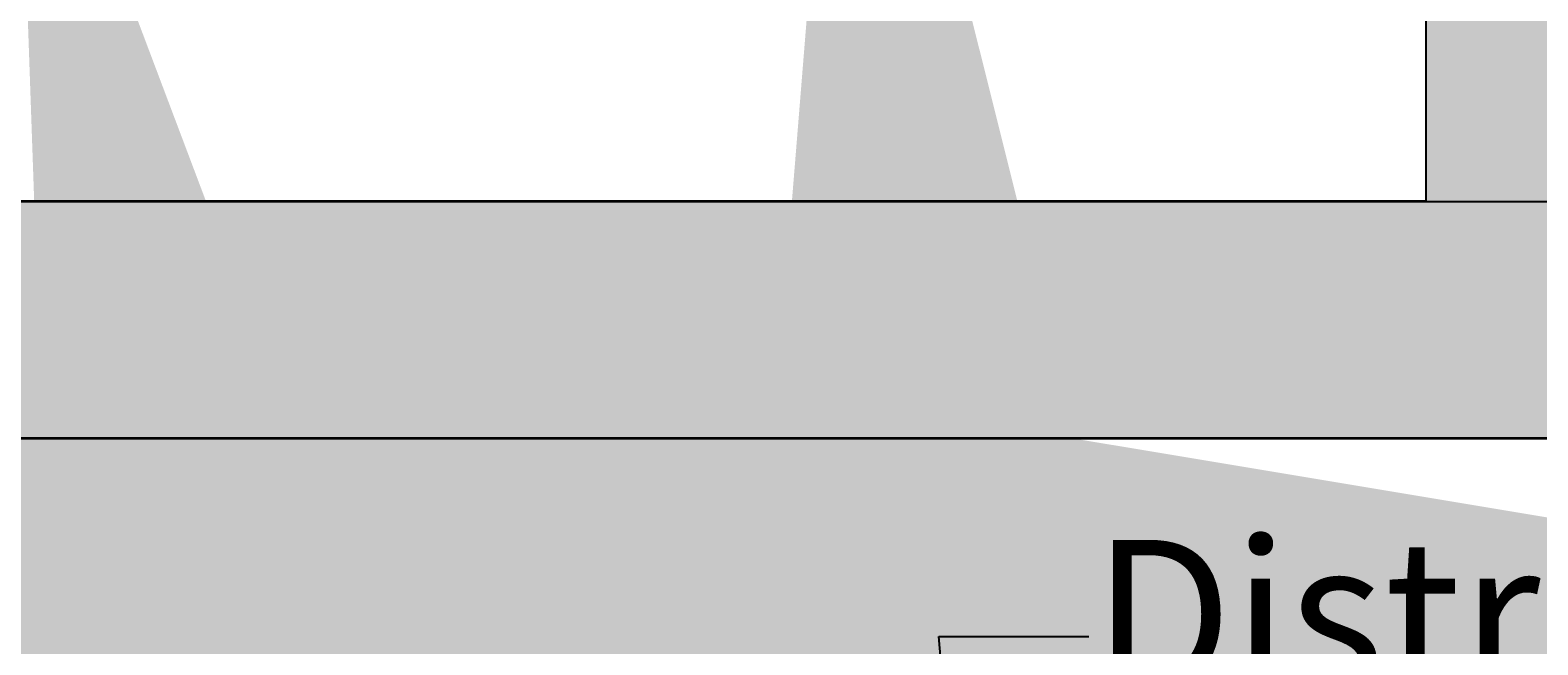
# Model space of a CAD drawing. Units: millimetres. Extents: x -22994 to 29398, y -19990 to 20176.
# Tile 13 of 135: x 58 to 99, y 5 to 21. Entities that reach past the tile are written whole.
import ezdxf
from ezdxf import colors
from ezdxf.entities.mleader import LeaderData, LeaderLine
from ezdxf.math import Vec2, Vec3

# ---------------------------------------------------------------- set-up
doc = ezdxf.new("R2010")
doc.units = ezdxf.units.MM
doc.header["$MEASUREMENT"] = 0
for name, color, linetype, lineweight in [('M-ANNO-TEXT', 7, 'Continuous', 25), ('M-DIMS', 2, 'Continuous', 18), ('M-EQPM', 7, 'Continuous', 25), ('M-EQPM-PATT', 7, 'Continuous', 18), ('S-FNDN', 7, 'Continuous', 35)]:
    doc.layers.add(name, color=color, linetype=linetype, lineweight=lineweight)
doc.styles.get("Standard").update_dxf_attribs({"font": 'arial.ttf'})
doc.dimstyles.get("Standard").update_dxf_attribs({"dimtxt": 0.18, "dimasz": 10000, "dimexe": 0.18, "dimexo": 0.0625, "dimgap": 0.09, "dimtad": 0, "dimtih": 1, "dimtoh": 1, "dimdec": 0, "dimzin": 0, "dimdsep": 46, "dimtxsty": 'Standard', "dimcen": 0.09, "dimadec": 0, "dimazin": 0, "dimtfac": 1, "dimtdec": 0, "dimtofl": 0, "dimtmove": 0, "dimatfit": 3, "dimfxl": 1, "dimtolj": 1, "dimtzin": 0, "dimlwd": 30, "dimarcsym": 0})

# ---------------------------------------------------------------- blocks, each defined once
blk = doc.blocks.new('*D2')
at = {"layer": 'Defpoints', "color": 0, "transparency": 16777216}
for p in [(6.677, 10.271), (290.852, 10.271), (290.852, -5.079)]:
    blk.add_point(p, dxfattribs=at)
at = {"layer": 'M-DIMS', "color": 0, "lineweight": -2, "transparency": 16777216}
for p, q in [((6.677, 10.209), (6.677, -5.259)), ((290.852, 10.209), (290.852, -5.259))]:
    blk.add_line(p, q, dxfattribs=at)
at = {"layer": 'M-DIMS', "color": 0, "lineweight": 30, "transparency": 16777216}
for p, q in [((-9993.323, -5.079), (-19993.323, -5.079)), ((10290.852, -5.079), (20290.852, -5.079))]:
    blk.add_line(p, q, dxfattribs=at)
at = {"layer": 'M-DIMS', "color": 0, "transparency": 16777216}
for points in [[(-9993.323, 1661.588), (-9993.323, -1671.745), (6.677, -5.079)], [(10290.852, 1661.588), (10290.852, -1671.745), (290.852, -5.079)]]:
    blk.add_solid(points, dxfattribs=at)
at = {"layer": 'M-DIMS', "color": 0, "transparency": 16777216, "insert": (148.765, -5.079), "char_height": 0.18, "attachment_point": 5}
blk.add_mtext('\\A1;284.2', dxfattribs=at)
blk = doc.blocks.new('*D3')
at = {"layer": 'Defpoints', "color": 0, "transparency": 16777216}
for p in [(110.265, 204.165), (110.265, 176.366), (95.833, 127.967)]:
    blk.add_point(p, dxfattribs=at)
at = {"layer": 'M-DIMS', "color": 0, "lineweight": 30, "transparency": 16777216}
for p, q in [((-9904.167, 204.165), (-19904.167, 204.165)), ((10110.265, 204.165), (20110.265, 204.165))]:
    blk.add_line(p, q, dxfattribs=at)
at = {"layer": 'M-DIMS', "color": 0, "lineweight": -2, "transparency": 16777216}
for p, q in [((95.833, 128.03), (95.833, 204.345)), ((110.265, 176.429), (110.265, 204.345))]:
    blk.add_line(p, q, dxfattribs=at)
at = {"layer": 'M-DIMS', "color": 0, "transparency": 16777216}
for points in [[(-9904.167, 1870.832), (-9904.167, -1462.501), (95.833, 204.165)], [(10110.265, 1870.832), (10110.265, -1462.501), (110.265, 204.165)]]:
    blk.add_solid(points, dxfattribs=at)
at = {"layer": 'M-DIMS', "color": 0, "transparency": 16777216, "insert": (103.049, 204.165), "char_height": 0.18, "attachment_point": 5}
blk.add_mtext('\\A1;14.432', dxfattribs=at)
blk = doc.blocks.new('*D4')
at = {"layer": 'Defpoints', "color": 0, "transparency": 16777216}
for p in [(116.265, 204.165), (110.265, 176.366), (116.265, 176.366)]:
    blk.add_point(p, dxfattribs=at)
at = {"layer": 'M-DIMS', "color": 0, "lineweight": 30, "transparency": 16777216}
for p, q in [((-9889.735, 204.165), (-19889.735, 204.165)), ((10116.265, 204.165), (20116.265, 204.165))]:
    blk.add_line(p, q, dxfattribs=at)
at = {"layer": 'M-DIMS', "color": 0, "lineweight": -2, "transparency": 16777216}
for p, q in [((110.265, 176.429), (110.265, 204.345)), ((116.265, 176.429), (116.265, 204.345))]:
    blk.add_line(p, q, dxfattribs=at)
at = {"layer": 'M-DIMS', "color": 0, "transparency": 16777216}
for points in [[(-9889.735, 1870.832), (-9889.735, -1462.501), (110.265, 204.165)], [(10116.265, 1870.832), (10116.265, -1462.501), (116.265, 204.165)]]:
    blk.add_solid(points, dxfattribs=at)
at = {"layer": 'M-DIMS', "color": 0, "transparency": 16777216, "insert": (113.265, 204.165), "char_height": 0.18, "attachment_point": 5}
blk.add_mtext('\\A1;6', dxfattribs=at)
blk = doc.blocks.new('*D5')
at = {"layer": 'Defpoints', "color": 0, "transparency": 16777216}
for p in [(181.265, 204.165), (116.265, 176.366), (181.265, 176.366)]:
    blk.add_point(p, dxfattribs=at)
at = {"layer": 'M-DIMS', "color": 0, "lineweight": 30, "transparency": 16777216}
for p, q in [((-9883.735, 204.165), (-19883.735, 204.165)), ((10181.265, 204.165), (20181.265, 204.165))]:
    blk.add_line(p, q, dxfattribs=at)
at = {"layer": 'M-DIMS', "color": 0, "lineweight": -2, "transparency": 16777216}
for p, q in [((116.265, 176.429), (116.265, 204.345)), ((181.265, 176.429), (181.265, 204.345))]:
    blk.add_line(p, q, dxfattribs=at)
at = {"layer": 'M-DIMS', "color": 0, "transparency": 16777216}
for points in [[(-9883.735, 1870.832), (-9883.735, -1462.501), (116.265, 204.165)], [(10181.265, 1870.832), (10181.265, -1462.501), (181.265, 204.165)]]:
    blk.add_solid(points, dxfattribs=at)
at = {"layer": 'M-DIMS', "color": 0, "transparency": 16777216, "insert": (148.765, 204.165), "char_height": 0.18, "attachment_point": 5}
blk.add_mtext('\\A1;65', dxfattribs=at)
blk = doc.blocks.new('*D6')
at = {"layer": 'Defpoints', "color": 0, "transparency": 16777216}
for p in [(187.265, 204.165), (181.265, 176.366), (187.265, 176.366)]:
    blk.add_point(p, dxfattribs=at)
at = {"layer": 'M-DIMS', "color": 0, "lineweight": 30, "transparency": 16777216}
for p, q in [((-9818.735, 204.165), (-19818.735, 204.165)), ((10187.265, 204.165), (20187.265, 204.165))]:
    blk.add_line(p, q, dxfattribs=at)
at = {"layer": 'M-DIMS', "color": 0, "lineweight": -2, "transparency": 16777216}
for p, q in [((181.265, 176.429), (181.265, 204.345)), ((187.265, 176.429), (187.265, 204.345))]:
    blk.add_line(p, q, dxfattribs=at)
at = {"layer": 'M-DIMS', "color": 0, "transparency": 16777216}
for points in [[(-9818.735, 1870.832), (-9818.735, -1462.501), (181.265, 204.165)], [(10187.265, 1870.832), (10187.265, -1462.501), (187.265, 204.165)]]:
    blk.add_solid(points, dxfattribs=at)
at = {"layer": 'M-DIMS', "color": 0, "transparency": 16777216, "insert": (184.265, 204.165), "char_height": 0.18, "attachment_point": 5}
blk.add_mtext('\\A1;6', dxfattribs=at)
blk = doc.blocks.new('*D7')
at = {"layer": 'Defpoints', "color": 0, "transparency": 16777216}
for p in [(201.697, 204.165), (187.265, 176.366), (201.697, 127.967)]:
    blk.add_point(p, dxfattribs=at)
at = {"layer": 'M-DIMS', "color": 0, "lineweight": 30, "transparency": 16777216}
for p, q in [((-9812.735, 204.165), (-19812.735, 204.165)), ((10201.697, 204.165), (20201.697, 204.165))]:
    blk.add_line(p, q, dxfattribs=at)
at = {"layer": 'M-DIMS', "color": 0, "lineweight": -2, "transparency": 16777216}
for p, q in [((187.265, 176.429), (187.265, 204.345)), ((201.697, 128.03), (201.697, 204.345))]:
    blk.add_line(p, q, dxfattribs=at)
at = {"layer": 'M-DIMS', "color": 0, "transparency": 16777216}
for points in [[(-9812.735, 1870.832), (-9812.735, -1462.501), (187.265, 204.165)], [(10201.697, 1870.832), (10201.697, -1462.501), (201.697, 204.165)]]:
    blk.add_solid(points, dxfattribs=at)
at = {"layer": 'M-DIMS', "color": 0, "transparency": 16777216, "insert": (194.481, 204.165), "char_height": 0.18, "attachment_point": 5}
blk.add_mtext('\\A1;14.432', dxfattribs=at)
blk = doc.blocks.new('*D8')
at = {"layer": 'Defpoints', "color": 0, "transparency": 16777216}
for p in [(227.648, 204.165), (227.648, 146.73), (201.697, 127.967)]:
    blk.add_point(p, dxfattribs=at)
at = {"layer": 'M-DIMS', "color": 0, "lineweight": 30, "transparency": 16777216}
for p, q in [((-9798.303, 204.165), (-19798.303, 204.165)), ((10227.648, 204.165), (20227.648, 204.165))]:
    blk.add_line(p, q, dxfattribs=at)
at = {"layer": 'M-DIMS', "color": 0, "lineweight": -2, "transparency": 16777216}
for p, q in [((201.697, 128.03), (201.697, 204.345)), ((227.648, 146.792), (227.648, 204.345))]:
    blk.add_line(p, q, dxfattribs=at)
at = {"layer": 'M-DIMS', "color": 0, "transparency": 16777216}
for points in [[(-9798.303, 1870.832), (-9798.303, -1462.501), (201.697, 204.165)], [(10227.648, 1870.832), (10227.648, -1462.501), (227.648, 204.165)]]:
    blk.add_solid(points, dxfattribs=at)
at = {"layer": 'M-DIMS', "color": 0, "transparency": 16777216, "insert": (214.673, 204.165), "char_height": 0.18, "attachment_point": 5}
blk.add_mtext('\\A1;25.95', dxfattribs=at)
blk = doc.blocks.new('*D9')
at = {"layer": 'Defpoints', "color": 0, "transparency": 16777216}
for p in [(187.265, 176.366), (306.202, 176.366), (290.852, 10.271)]:
    blk.add_point(p, dxfattribs=at)
at = {"layer": 'M-DIMS', "color": 0, "lineweight": 30, "transparency": 16777216}
for p, q in [((306.202, 10176.366), (306.202, 20176.366)), ((306.202, -9989.729), (306.202, -19989.729))]:
    blk.add_line(p, q, dxfattribs=at)
at = {"layer": 'M-DIMS', "color": 0, "lineweight": -2, "transparency": 16777216}
for p, q in [((187.327, 176.366), (306.382, 176.366)), ((290.915, 10.271), (306.382, 10.271))]:
    blk.add_line(p, q, dxfattribs=at)
at = {"layer": 'M-DIMS', "color": 0, "transparency": 16777216}
for points in [[(-1360.465, 10176.366), (1972.869, 10176.366), (306.202, 176.366)], [(-1360.465, -9989.729), (1972.869, -9989.729), (306.202, 10.271)]]:
    blk.add_solid(points, dxfattribs=at)
at = {"layer": 'M-DIMS', "color": 0, "transparency": 16777216, "insert": (306.202, 93.319), "char_height": 0.18, "attachment_point": 5}
blk.add_mtext('\\A1;166.1', dxfattribs=at)
blk = doc.blocks.new('*D10')
at = {"layer": 'Defpoints', "color": 0, "transparency": 16777216}
for p in [(125.65, 136.071), (133.346, 136.071), (133.346, -5.079)]:
    blk.add_point(p, dxfattribs=at)
at = {"layer": 'M-DIMS', "color": 0, "lineweight": -2, "transparency": 16777216}
for p, q in [((125.65, 136.009), (125.65, -5.259)), ((133.346, 136.009), (133.346, -5.259))]:
    blk.add_line(p, q, dxfattribs=at)
at = {"layer": 'M-DIMS', "color": 0, "lineweight": 30, "transparency": 16777216}
for p, q in [((-9874.35, -5.079), (-19874.35, -5.079)), ((10133.346, -5.079), (20133.346, -5.079))]:
    blk.add_line(p, q, dxfattribs=at)
at = {"layer": 'M-DIMS', "color": 0, "transparency": 16777216}
for points in [[(-9874.35, 1661.588), (-9874.35, -1671.745), (125.65, -5.079)], [(10133.346, 1661.588), (10133.346, -1671.745), (133.346, -5.079)]]:
    blk.add_solid(points, dxfattribs=at)
at = {"layer": 'M-DIMS', "color": 0, "transparency": 16777216, "insert": (129.498, -5.079), "char_height": 0.18, "attachment_point": 5}
blk.add_mtext('\\A1;7.696', dxfattribs=at)
blk = doc.blocks.new('*D11')
at = {"layer": 'Defpoints', "color": 0, "transparency": 16777216}
for p in [(133.346, 136.071), (135.65, 136.071), (135.65, -5.079)]:
    blk.add_point(p, dxfattribs=at)
at = {"layer": 'M-DIMS', "color": 0, "lineweight": -2, "transparency": 16777216}
for p, q in [((133.346, 136.009), (133.346, -5.259)), ((135.65, 136.009), (135.65, -5.259))]:
    blk.add_line(p, q, dxfattribs=at)
at = {"layer": 'M-DIMS', "color": 0, "lineweight": 30, "transparency": 16777216}
for p, q in [((-9866.654, -5.079), (-19866.654, -5.079)), ((10135.65, -5.079), (20135.65, -5.079))]:
    blk.add_line(p, q, dxfattribs=at)
at = {"layer": 'M-DIMS', "color": 0, "transparency": 16777216}
for points in [[(-9866.654, 1661.588), (-9866.654, -1671.745), (133.346, -5.079)], [(10135.65, 1661.588), (10135.65, -1671.745), (135.65, -5.079)]]:
    blk.add_solid(points, dxfattribs=at)
at = {"layer": 'M-DIMS', "color": 0, "transparency": 16777216, "insert": (134.498, -5.079), "char_height": 0.18, "attachment_point": 5}
blk.add_mtext('\\A1;2.304', dxfattribs=at)
blk = doc.blocks.new('*D12')
at = {"layer": 'Defpoints', "color": 0, "transparency": 16777216}
for p in [(135.65, 136.071), (145.65, 136.071), (145.65, -5.079)]:
    blk.add_point(p, dxfattribs=at)
at = {"layer": 'M-DIMS', "color": 0, "lineweight": -2, "transparency": 16777216}
for p, q in [((135.65, 136.009), (135.65, -5.259)), ((145.65, 136.009), (145.65, -5.259))]:
    blk.add_line(p, q, dxfattribs=at)
at = {"layer": 'M-DIMS', "color": 0, "lineweight": 30, "transparency": 16777216}
for p, q in [((-9864.35, -5.079), (-19864.35, -5.079)), ((10145.65, -5.079), (20145.65, -5.079))]:
    blk.add_line(p, q, dxfattribs=at)
at = {"layer": 'M-DIMS', "color": 0, "transparency": 16777216}
for points in [[(-9864.35, 1661.588), (-9864.35, -1671.745), (135.65, -5.079)], [(10145.65, 1661.588), (10145.65, -1671.745), (145.65, -5.079)]]:
    blk.add_solid(points, dxfattribs=at)
at = {"layer": 'M-DIMS', "color": 0, "transparency": 16777216, "insert": (140.65, -5.079), "char_height": 0.18, "attachment_point": 5}
blk.add_mtext('\\A1;10', dxfattribs=at)
blk = doc.blocks.new('*D13')
at = {"layer": 'Defpoints', "color": 0, "transparency": 16777216}
for p in [(145.65, 136.071), (155.65, 136.071), (155.65, -5.079)]:
    blk.add_point(p, dxfattribs=at)
at = {"layer": 'M-DIMS', "color": 0, "lineweight": -2, "transparency": 16777216}
for p, q in [((145.65, 136.009), (145.65, -5.259)), ((155.65, 136.009), (155.65, -5.259))]:
    blk.add_line(p, q, dxfattribs=at)
at = {"layer": 'M-DIMS', "color": 0, "lineweight": 30, "transparency": 16777216}
for p, q in [((-9854.35, -5.079), (-19854.35, -5.079)), ((10155.65, -5.079), (20155.65, -5.079))]:
    blk.add_line(p, q, dxfattribs=at)
at = {"layer": 'M-DIMS', "color": 0, "transparency": 16777216}
for points in [[(-9854.35, 1661.588), (-9854.35, -1671.745), (145.65, -5.079)], [(10155.65, 1661.588), (10155.65, -1671.745), (155.65, -5.079)]]:
    blk.add_solid(points, dxfattribs=at)
at = {"layer": 'M-DIMS', "color": 0, "transparency": 16777216, "insert": (150.65, -5.079), "char_height": 0.18, "attachment_point": 5}
blk.add_mtext('\\A1;10', dxfattribs=at)
blk = doc.blocks.new('*D14')
at = {"layer": 'Defpoints', "color": 0, "transparency": 16777216}
for p in [(155.65, 136.071), (165.65, 136.071), (165.65, -5.079)]:
    blk.add_point(p, dxfattribs=at)
at = {"layer": 'M-DIMS', "color": 0, "lineweight": -2, "transparency": 16777216}
for p, q in [((155.65, 136.009), (155.65, -5.259)), ((165.65, 136.009), (165.65, -5.259))]:
    blk.add_line(p, q, dxfattribs=at)
at = {"layer": 'M-DIMS', "color": 0, "lineweight": 30, "transparency": 16777216}
for p, q in [((-9844.35, -5.079), (-19844.35, -5.079)), ((10165.65, -5.079), (20165.65, -5.079))]:
    blk.add_line(p, q, dxfattribs=at)
at = {"layer": 'M-DIMS', "color": 0, "transparency": 16777216}
for points in [[(-9844.35, 1661.588), (-9844.35, -1671.745), (155.65, -5.079)], [(10165.65, 1661.588), (10165.65, -1671.745), (165.65, -5.079)]]:
    blk.add_solid(points, dxfattribs=at)
at = {"layer": 'M-DIMS', "color": 0, "transparency": 16777216, "insert": (160.65, -5.079), "char_height": 0.18, "attachment_point": 5}
blk.add_mtext('\\A1;10', dxfattribs=at)
blk = doc.blocks.new('*D15')
at = {"layer": 'Defpoints', "color": 0, "transparency": 16777216}
for p in [(173.346, 154.788), (173.346, 136.071), (306.202, 136.071)]:
    blk.add_point(p, dxfattribs=at)
at = {"layer": 'M-DIMS', "color": 0, "lineweight": 30, "transparency": 16777216}
for p, q in [((306.202, 10154.788), (306.202, 20154.788)), ((306.202, -9863.929), (306.202, -19863.929))]:
    blk.add_line(p, q, dxfattribs=at)
at = {"layer": 'M-DIMS', "color": 0, "lineweight": -2, "transparency": 16777216}
for p, q in [((173.408, 154.788), (306.382, 154.788)), ((173.408, 136.071), (306.382, 136.071))]:
    blk.add_line(p, q, dxfattribs=at)
at = {"layer": 'M-DIMS', "color": 0, "transparency": 16777216}
for points in [[(-1360.465, 10154.788), (1972.869, 10154.788), (306.202, 154.788)], [(-1360.465, -9863.929), (1972.869, -9863.929), (306.202, 136.071)]]:
    blk.add_solid(points, dxfattribs=at)
at = {"layer": 'M-DIMS', "color": 0, "transparency": 16777216, "insert": (306.202, 145.43), "char_height": 0.18, "attachment_point": 5}
blk.add_mtext('\\A1;18.717', dxfattribs=at)
blk = doc.blocks.new('*D16')
at = {"layer": 'Defpoints', "color": 0, "transparency": 16777216}
for p in [(120.17, 204.165), (110.466, 48.035), (120.17, 48.035)]:
    blk.add_point(p, dxfattribs=at)
at = {"layer": 'M-DIMS', "color": 0, "lineweight": 30, "transparency": 16777216}
for p, q in [((-9889.534, 204.165), (-19889.534, 204.165)), ((10120.17, 204.165), (20120.17, 204.165))]:
    blk.add_line(p, q, dxfattribs=at)
at = {"layer": 'M-DIMS', "color": 0, "lineweight": -2, "transparency": 16777216}
for p, q in [((110.466, 48.097), (110.466, 204.345)), ((120.17, 48.097), (120.17, 204.345))]:
    blk.add_line(p, q, dxfattribs=at)
at = {"layer": 'M-DIMS', "color": 0, "transparency": 16777216}
for points in [[(-9889.534, 1870.832), (-9889.534, -1462.501), (110.466, 204.165)], [(10120.17, 1870.832), (10120.17, -1462.501), (120.17, 204.165)]]:
    blk.add_solid(points, dxfattribs=at)
at = {"layer": 'M-DIMS', "color": 0, "transparency": 16777216, "insert": (115.318, 204.165), "char_height": 0.18, "attachment_point": 5}
blk.add_mtext('\\A1;9.704', dxfattribs=at)
blk = doc.blocks.new('*D17')
at = {"layer": 'Defpoints', "color": 0, "transparency": 16777216}
for p in [(126.17, 204.165), (120.17, 48.035), (126.17, 48.035)]:
    blk.add_point(p, dxfattribs=at)
at = {"layer": 'M-DIMS', "color": 0, "lineweight": 30, "transparency": 16777216}
for p, q in [((-9879.83, 204.165), (-19879.83, 204.165)), ((10126.17, 204.165), (20126.17, 204.165))]:
    blk.add_line(p, q, dxfattribs=at)
at = {"layer": 'M-DIMS', "color": 0, "lineweight": -2, "transparency": 16777216}
for p, q in [((120.17, 48.097), (120.17, 204.345)), ((126.17, 48.097), (126.17, 204.345))]:
    blk.add_line(p, q, dxfattribs=at)
at = {"layer": 'M-DIMS', "color": 0, "transparency": 16777216}
for points in [[(-9879.83, 1870.832), (-9879.83, -1462.501), (120.17, 204.165)], [(10126.17, 1870.832), (10126.17, -1462.501), (126.17, 204.165)]]:
    blk.add_solid(points, dxfattribs=at)
at = {"layer": 'M-DIMS', "color": 0, "transparency": 16777216, "insert": (123.17, 204.165), "char_height": 0.18, "attachment_point": 5}
blk.add_mtext('\\A1;6', dxfattribs=at)
blk = doc.blocks.new('*D18')
at = {"layer": 'Defpoints', "color": 0, "transparency": 16777216}
for p in [(132.17, 204.165), (126.17, 48.035), (132.17, 48.035)]:
    blk.add_point(p, dxfattribs=at)
at = {"layer": 'M-DIMS', "color": 0, "lineweight": 30, "transparency": 16777216}
for p, q in [((-9873.83, 204.165), (-19873.83, 204.165)), ((10132.17, 204.165), (20132.17, 204.165))]:
    blk.add_line(p, q, dxfattribs=at)
at = {"layer": 'M-DIMS', "color": 0, "lineweight": -2, "transparency": 16777216}
for p, q in [((126.17, 48.097), (126.17, 204.345)), ((132.17, 48.097), (132.17, 204.345))]:
    blk.add_line(p, q, dxfattribs=at)
at = {"layer": 'M-DIMS', "color": 0, "transparency": 16777216}
for points in [[(-9873.83, 1870.832), (-9873.83, -1462.501), (126.17, 204.165)], [(10132.17, 1870.832), (10132.17, -1462.501), (132.17, 204.165)]]:
    blk.add_solid(points, dxfattribs=at)
at = {"layer": 'M-DIMS', "color": 0, "transparency": 16777216, "insert": (129.17, 204.165), "char_height": 0.18, "attachment_point": 5}
blk.add_mtext('\\A1;6', dxfattribs=at)
blk = doc.blocks.new('*D19')
at = {"layer": 'Defpoints', "color": 0, "transparency": 16777216}
for p in [(138.17, 204.165), (132.17, 48.035), (138.17, 48.035)]:
    blk.add_point(p, dxfattribs=at)
at = {"layer": 'M-DIMS', "color": 0, "lineweight": 30, "transparency": 16777216}
for p, q in [((-9867.83, 204.165), (-19867.83, 204.165)), ((10138.17, 204.165), (20138.17, 204.165))]:
    blk.add_line(p, q, dxfattribs=at)
at = {"layer": 'M-DIMS', "color": 0, "lineweight": -2, "transparency": 16777216}
for p, q in [((132.17, 48.097), (132.17, 204.345)), ((138.17, 48.097), (138.17, 204.345))]:
    blk.add_line(p, q, dxfattribs=at)
at = {"layer": 'M-DIMS', "color": 0, "transparency": 16777216}
for points in [[(-9867.83, 1870.832), (-9867.83, -1462.501), (132.17, 204.165)], [(10138.17, 1870.832), (10138.17, -1462.501), (138.17, 204.165)]]:
    blk.add_solid(points, dxfattribs=at)
at = {"layer": 'M-DIMS', "color": 0, "transparency": 16777216, "insert": (135.17, 204.165), "char_height": 0.18, "attachment_point": 5}
blk.add_mtext('\\A1;6', dxfattribs=at)
blk = doc.blocks.new('*D20')
at = {"layer": 'Defpoints', "color": 0, "transparency": 16777216}
for p in [(144.17, 204.165), (138.17, 48.035), (144.17, 48.035)]:
    blk.add_point(p, dxfattribs=at)
at = {"layer": 'M-DIMS', "color": 0, "lineweight": 30, "transparency": 16777216}
for p, q in [((-9861.83, 204.165), (-19861.83, 204.165)), ((10144.17, 204.165), (20144.17, 204.165))]:
    blk.add_line(p, q, dxfattribs=at)
at = {"layer": 'M-DIMS', "color": 0, "lineweight": -2, "transparency": 16777216}
for p, q in [((138.17, 48.097), (138.17, 204.345)), ((144.17, 48.097), (144.17, 204.345))]:
    blk.add_line(p, q, dxfattribs=at)
at = {"layer": 'M-DIMS', "color": 0, "transparency": 16777216}
for points in [[(-9861.83, 1870.832), (-9861.83, -1462.501), (138.17, 204.165)], [(10144.17, 1870.832), (10144.17, -1462.501), (144.17, 204.165)]]:
    blk.add_solid(points, dxfattribs=at)
at = {"layer": 'M-DIMS', "color": 0, "transparency": 16777216, "insert": (141.17, 204.165), "char_height": 0.18, "attachment_point": 5}
blk.add_mtext('\\A1;6', dxfattribs=at)
blk = doc.blocks.new('*D21')
at = {"layer": 'Defpoints', "color": 0, "transparency": 16777216}
for p in [(149.116, 204.165), (144.17, 48.035), (149.116, 48.035)]:
    blk.add_point(p, dxfattribs=at)
at = {"layer": 'M-DIMS', "color": 0, "lineweight": 30, "transparency": 16777216}
for p, q in [((-9855.83, 204.165), (-19855.83, 204.165)), ((10149.116, 204.165), (20149.116, 204.165))]:
    blk.add_line(p, q, dxfattribs=at)
at = {"layer": 'M-DIMS', "color": 0, "lineweight": -2, "transparency": 16777216}
for p, q in [((144.17, 48.097), (144.17, 204.345)), ((149.116, 48.097), (149.116, 204.345))]:
    blk.add_line(p, q, dxfattribs=at)
at = {"layer": 'M-DIMS', "color": 0, "transparency": 16777216}
for points in [[(-9855.83, 1870.832), (-9855.83, -1462.501), (144.17, 204.165)], [(10149.116, 1870.832), (10149.116, -1462.501), (149.116, 204.165)]]:
    blk.add_solid(points, dxfattribs=at)
at = {"layer": 'M-DIMS', "color": 0, "transparency": 16777216, "insert": (146.643, 204.165), "char_height": 0.18, "attachment_point": 5}
blk.add_mtext('\\A1;4.945', dxfattribs=at)
blk = doc.blocks.new('*D22')
at = {"layer": 'Defpoints', "color": 0, "transparency": 16777216}
for p in [(149.116, 30.99), (155.116, 30.99), (155.116, -5.079)]:
    blk.add_point(p, dxfattribs=at)
at = {"layer": 'M-DIMS', "color": 0, "lineweight": -2, "transparency": 16777216}
for p, q in [((149.116, 30.927), (149.116, -5.259)), ((155.116, 30.927), (155.116, -5.259))]:
    blk.add_line(p, q, dxfattribs=at)
at = {"layer": 'M-DIMS', "color": 0, "lineweight": 30, "transparency": 16777216}
for p, q in [((-9850.884, -5.079), (-19850.884, -5.079)), ((10155.116, -5.079), (20155.116, -5.079))]:
    blk.add_line(p, q, dxfattribs=at)
at = {"layer": 'M-DIMS', "color": 0, "transparency": 16777216}
for points in [[(-9850.884, 1661.588), (-9850.884, -1671.745), (149.116, -5.079)], [(10155.116, 1661.588), (10155.116, -1671.745), (155.116, -5.079)]]:
    blk.add_solid(points, dxfattribs=at)
at = {"layer": 'M-DIMS', "color": 0, "transparency": 16777216, "insert": (152.116, -5.079), "char_height": 0.18, "attachment_point": 5}
blk.add_mtext('\\A1;6', dxfattribs=at)
blk = doc.blocks.new('*D23')
at = {"layer": 'Defpoints', "color": 0, "transparency": 16777216}
for p in [(155.116, 30.99), (161.116, 30.99), (161.116, -5.079)]:
    blk.add_point(p, dxfattribs=at)
at = {"layer": 'M-DIMS', "color": 0, "lineweight": -2, "transparency": 16777216}
for p, q in [((155.116, 30.927), (155.116, -5.259)), ((161.116, 30.927), (161.116, -5.259))]:
    blk.add_line(p, q, dxfattribs=at)
at = {"layer": 'M-DIMS', "color": 0, "lineweight": 30, "transparency": 16777216}
for p, q in [((-9844.884, -5.079), (-19844.884, -5.079)), ((10161.116, -5.079), (20161.116, -5.079))]:
    blk.add_line(p, q, dxfattribs=at)
at = {"layer": 'M-DIMS', "color": 0, "transparency": 16777216}
for points in [[(-9844.884, 1661.588), (-9844.884, -1671.745), (155.116, -5.079)], [(10161.116, 1661.588), (10161.116, -1671.745), (161.116, -5.079)]]:
    blk.add_solid(points, dxfattribs=at)
at = {"layer": 'M-DIMS', "color": 0, "transparency": 16777216, "insert": (158.116, -5.079), "char_height": 0.18, "attachment_point": 5}
blk.add_mtext('\\A1;6', dxfattribs=at)
blk = doc.blocks.new('*D24')
at = {"layer": 'Defpoints', "color": 0, "transparency": 16777216}
for p in [(161.116, 30.99), (166.439, 30.99), (166.439, -5.079)]:
    blk.add_point(p, dxfattribs=at)
at = {"layer": 'M-DIMS', "color": 0, "lineweight": -2, "transparency": 16777216}
for p, q in [((161.116, 30.927), (161.116, -5.259)), ((166.439, 30.927), (166.439, -5.259))]:
    blk.add_line(p, q, dxfattribs=at)
at = {"layer": 'M-DIMS', "color": 0, "lineweight": 30, "transparency": 16777216}
for p, q in [((-9838.884, -5.079), (-19838.884, -5.079)), ((10166.439, -5.079), (20166.439, -5.079))]:
    blk.add_line(p, q, dxfattribs=at)
at = {"layer": 'M-DIMS', "color": 0, "transparency": 16777216}
for points in [[(-9838.884, 1661.588), (-9838.884, -1671.745), (161.116, -5.079)], [(10166.439, 1661.588), (10166.439, -1671.745), (166.439, -5.079)]]:
    blk.add_solid(points, dxfattribs=at)
at = {"layer": 'M-DIMS', "color": 0, "transparency": 16777216, "insert": (163.777, -5.079), "char_height": 0.18, "attachment_point": 5}
blk.add_mtext('\\A1;5.323', dxfattribs=at)
blk = doc.blocks.new('*D25')
at = {"layer": 'Defpoints', "color": 0, "transparency": 16777216}
for p in [(166.439, 30.99), (172.439, 30.99), (172.439, -5.079)]:
    blk.add_point(p, dxfattribs=at)
at = {"layer": 'M-DIMS', "color": 0, "lineweight": -2, "transparency": 16777216}
for p, q in [((166.439, 30.927), (166.439, -5.259)), ((172.439, 30.927), (172.439, -5.259))]:
    blk.add_line(p, q, dxfattribs=at)
at = {"layer": 'M-DIMS', "color": 0, "lineweight": 30, "transparency": 16777216}
for p, q in [((-9833.561, -5.079), (-19833.561, -5.079)), ((10172.439, -5.079), (20172.439, -5.079))]:
    blk.add_line(p, q, dxfattribs=at)
at = {"layer": 'M-DIMS', "color": 0, "transparency": 16777216}
for points in [[(-9833.561, 1661.588), (-9833.561, -1671.745), (166.439, -5.079)], [(10172.439, 1661.588), (10172.439, -1671.745), (172.439, -5.079)]]:
    blk.add_solid(points, dxfattribs=at)
at = {"layer": 'M-DIMS', "color": 0, "transparency": 16777216, "insert": (169.439, -5.079), "char_height": 0.18, "attachment_point": 5}
blk.add_mtext('\\A1;6', dxfattribs=at)
blk = doc.blocks.new('*D26')
at = {"layer": 'Defpoints', "color": 0, "transparency": 16777216}
for p in [(172.439, 30.99), (178.439, 30.99), (178.439, -5.079)]:
    blk.add_point(p, dxfattribs=at)
at = {"layer": 'M-DIMS', "color": 0, "lineweight": -2, "transparency": 16777216}
for p, q in [((172.439, 30.927), (172.439, -5.259)), ((178.439, 30.927), (178.439, -5.259))]:
    blk.add_line(p, q, dxfattribs=at)
at = {"layer": 'M-DIMS', "color": 0, "lineweight": 30, "transparency": 16777216}
for p, q in [((-9827.561, -5.079), (-19827.561, -5.079)), ((10178.439, -5.079), (20178.439, -5.079))]:
    blk.add_line(p, q, dxfattribs=at)
at = {"layer": 'M-DIMS', "color": 0, "transparency": 16777216}
for points in [[(-9827.561, 1661.588), (-9827.561, -1671.745), (172.439, -5.079)], [(10178.439, 1661.588), (10178.439, -1671.745), (178.439, -5.079)]]:
    blk.add_solid(points, dxfattribs=at)
at = {"layer": 'M-DIMS', "color": 0, "transparency": 16777216, "insert": (175.439, -5.079), "char_height": 0.18, "attachment_point": 5}
blk.add_mtext('\\A1;6', dxfattribs=at)
blk = doc.blocks.new('*D27')
at = {"layer": 'Defpoints', "color": 0, "transparency": 16777216}
for p in [(178.439, 30.99), (188.117, 30.99), (188.117, -5.079)]:
    blk.add_point(p, dxfattribs=at)
at = {"layer": 'M-DIMS', "color": 0, "lineweight": -2, "transparency": 16777216}
for p, q in [((178.439, 30.927), (178.439, -5.259)), ((188.117, 30.927), (188.117, -5.259))]:
    blk.add_line(p, q, dxfattribs=at)
at = {"layer": 'M-DIMS', "color": 0, "lineweight": 30, "transparency": 16777216}
for p, q in [((-9821.561, -5.079), (-19821.561, -5.079)), ((10188.117, -5.079), (20188.117, -5.079))]:
    blk.add_line(p, q, dxfattribs=at)
at = {"layer": 'M-DIMS', "color": 0, "transparency": 16777216}
for points in [[(-9821.561, 1661.588), (-9821.561, -1671.745), (178.439, -5.079)], [(10188.117, 1661.588), (10188.117, -1671.745), (188.117, -5.079)]]:
    blk.add_solid(points, dxfattribs=at)
at = {"layer": 'M-DIMS', "color": 0, "transparency": 16777216, "insert": (183.278, -5.079), "char_height": 0.18, "attachment_point": 5}
blk.add_mtext('\\A1;9.679', dxfattribs=at)
blk = doc.blocks.new('*D28')
at = {"layer": 'Defpoints', "color": 0, "transparency": 16777216}
for p in [(188.117, 48.035), (306.202, 48.035), (188.117, 30.99)]:
    blk.add_point(p, dxfattribs=at)
at = {"layer": 'M-DIMS', "color": 0, "lineweight": 30, "transparency": 16777216}
for p, q in [((306.202, 10048.035), (306.202, 20048.035)), ((306.202, -9969.01), (306.202, -19969.01))]:
    blk.add_line(p, q, dxfattribs=at)
at = {"layer": 'M-DIMS', "color": 0, "lineweight": -2, "transparency": 16777216}
for p, q in [((188.18, 48.035), (306.382, 48.035)), ((188.18, 30.99), (306.382, 30.99))]:
    blk.add_line(p, q, dxfattribs=at)
at = {"layer": 'M-DIMS', "color": 0, "transparency": 16777216}
for points in [[(-1360.465, 10048.035), (1972.869, 10048.035), (306.202, 48.035)], [(-1360.465, -9969.01), (1972.869, -9969.01), (306.202, 30.99)]]:
    blk.add_solid(points, dxfattribs=at)
at = {"layer": 'M-DIMS', "color": 0, "transparency": 16777216, "insert": (306.202, 39.512), "char_height": 0.18, "attachment_point": 5}
blk.add_mtext('\\A1;17.045', dxfattribs=at)
blk = doc.blocks.new('*D29')
at = {"layer": 'Defpoints', "color": 0, "transparency": 16777216}
for p in [(36.801, 80.045), (64.03, 80.045)]:
    blk.add_point(p, dxfattribs=at)
at = {"layer": 'M-DIMS', "color": 0, "lineweight": -2, "transparency": 16777216}
for p, q in [((50.325, 80.045), (50.505, 80.045)), ((50.415, 79.955), (50.415, 80.135))]:
    blk.add_line(p, q, dxfattribs=at)
at = {"layer": 'M-DIMS', "color": 0, "lineweight": 30, "transparency": 16777216}
blk.add_line((20064.03, 80.03), (10064.03, 80.038), dxfattribs=at)
at = {"layer": 'M-DIMS', "color": 0, "transparency": 16777216}
blk.add_solid([(10064.031, 1746.704), (10064.028, -1586.629), (64.03, 80.045)], dxfattribs=at)
at = {"layer": 'M-DIMS', "color": 0, "transparency": 16777216, "insert": (20064.521, 80.03), "char_height": 0.18, "attachment_point": 5}
blk.add_mtext('\\A1;∅27.23', dxfattribs=at)
blk = doc.blocks.new('*D37')
at = {"layer": 'Defpoints', "color": 0, "transparency": 16777216}
for p in [(54.834, 118.615), (59.494, 118.614)]:
    blk.add_point(p, dxfattribs=at)
at = {"layer": 'M-DIMS', "color": 0, "lineweight": -2, "transparency": 16777216}
for p, q in [((57.074, 118.614), (57.254, 118.614)), ((57.164, 118.524), (57.164, 118.704))]:
    blk.add_line(p, q, dxfattribs=at)
at = {"layer": 'M-DIMS', "color": 0, "lineweight": 30, "transparency": 16777216}
blk.add_line((20059.493, 116.253), (10059.494, 117.434), dxfattribs=at)
at = {"layer": 'M-DIMS', "color": 0, "transparency": 16777216}
blk.add_solid([(10059.69, 1784.1), (10059.297, -1549.233), (59.494, 118.614)], dxfattribs=at)
at = {"layer": 'M-DIMS', "color": 0, "transparency": 16777216, "insert": (20059.985, 116.253), "char_height": 0.18, "attachment_point": 5}
blk.add_mtext('\\A1;∅4.659', dxfattribs=at)

msp = doc.modelspace()

# ---------------------------------------------------------------- hatches: boundary and pattern name
at = {"layer": 'M-EQPM-PATT'}
h = msp.add_hatch(color=256, dxfattribs=at)
h.set_gradient(color1=(205, 32, 39), color2=(205, 32, 39), tint=1)
h.paths.add_polyline_path([(116.2647, 150.3662), (116.2647, 170.3662), (116.2647, 176.3662), (110.2647, 176.3662), (110.2647, 152.0276), (95.8327, 127.967), (95.8327, 16.6063), (201.6967, 16.6063), (201.6967, 127.967), (187.2647, 152.0276), (187.2647, 176.3662), (181.2647, 176.3662), (181.2647, 170.3662), (181.2647, 150.3662), (195.6967, 126.3055), (195.6967, 22.6063), (101.8327, 22.6063), (101.8327, 126.3055)])
h.paths.add_polyline_path([(185.2208, 88.6347), (101.8327, 88.6347), (101.8327, 87.6347), (182.8066, 87.6347), (178.7313, 83.5594), (195.6967, 83.5594), (195.6967, 84.5594), (181.1455, 84.5594)], flags=17)
h.paths.add_polyline_path([(95.8327, 88.6347), (60.9779, 88.6347, -0.0228552), (61.7178, 87.6347), (95.8327, 87.6347)])
h.paths.add_polyline_path([(215.6212, 86.5189), (215.6212, 80.5999), (220.5095, 83.5594)])
h.paths.add_polyline_path([(215.6212, 84.5594), (201.6967, 84.5594), (201.6967, 83.5594), (215.6212, 83.5594)])
h.paths.add_polyline_path([(225.3978, 86.5189), (220.5095, 83.5594), (225.3978, 80.5999)])
h.paths.add_polyline_path([(231.6256, 84.5594), (225.3978, 84.5594), (225.3978, 83.5594), (231.6256, 83.5594)])
at = {"layer": 'S-FNDN'}
h = msp.add_hatch(color=256, dxfattribs=at)
h.set_gradient(color1=(241, 235, 31), color2=(244, 238, 81), tint=1, name='CYLINDER')
h.paths.add_polyline_path([(290.852, 16.6063), (201.6967, 16.6063), (95.8327, 16.6063), (81.8485, 16.6063), (82.3691, 10.2713), (290.852, 10.2713)])
h.paths.add_polyline_path([(81.8485, 16.6063), (60.8206, 16.6063), (62.0909, 10.2713), (82.3691, 10.2713)])
h.paths.add_polyline_path([(60.8206, 16.6063), (6.6773, 16.6063), (6.6773, 10.2713), (62.0909, 10.2713)])

# ---------------------------------------------------------------- linework, layer by layer
at = {"layer": 'M-EQPM'}
msp.add_lwpolyline([(110.2647, 176.3662), (110.2647, 152.0276), (95.8327, 127.967), (95.8327, 16.6063), (201.6967, 16.6063), (201.6967, 127.967), (187.2647, 152.0276), (187.2647, 176.3662)], close=True, dxfattribs=at)
at = {"layer": 'S-FNDN'}
msp.add_lwpolyline([(95.8327, 16.6063), (6.6773, 16.6063), (6.6773, 10.2713), (290.852, 10.2713), (290.852, 16.6063), (201.6967, 16.6063)], dxfattribs=at)

# ---------------------------------------------------------------- dimensions: what is measured, and where the dimension line sits
at = {"layer": 'M-DIMS'}
for base, p1, p2, override, picture, middle in [((306.202, 176.3662), (290.852, 10.2713), (187.2647, 176.3662), {"dimdec": 1, "dimlfac": 1, "dimrnd": 0, "dimzin": 0, "dimdsep": 46, "dimlunit": 2}, '*D9', (306.202, 93.3187)), ((306.202, 136.0713), (173.3459, 154.788), (173.3459, 136.0713), {"dimdec": 3, "dimlfac": 1, "dimrnd": 0, "dimzin": 0, "dimdsep": 46, "dimlunit": 2}, '*D15', (306.202, 145.4297)), ((306.202, 48.0349), (188.1175, 30.9895), (188.1175, 48.0349), {"dimdec": 3, "dimlfac": 1, "dimrnd": 0, "dimzin": 0, "dimdsep": 46, "dimlunit": 2}, '*D28', (306.202, 39.5122))]:
    dim = msp.add_linear_dim(base=base, p1=p1, p2=p2, angle=90, dimstyle='Standard', override=override, dxfattribs=at)
    dim.commit()
    dim.dimension.update_dxf_attribs({"geometry": picture, "text_midpoint": middle})
for base, p1, p2, override, picture, middle in [((110.2647, 204.1654), (95.8327, 127.967), (110.2647, 176.3662), {"dimdec": 3, "dimlfac": 1, "dimrnd": 0, "dimzin": 0, "dimdsep": 46, "dimlunit": 2}, '*D3', (103.0487, 204.1654)), ((116.2647, 204.1654), (110.2647, 176.3662), (116.2647, 176.3662), {"dimdec": 0, "dimlfac": 1, "dimrnd": 0, "dimzin": 0, "dimdsep": 46, "dimlunit": 2}, '*D4', (113.2647, 204.1654)), ((120.1702, 204.1654), (110.4658, 48.0349), (120.1702, 48.0349), {"dimdec": 3, "dimlfac": 1, "dimrnd": 0, "dimzin": 0, "dimdsep": 46, "dimlunit": 2}, '*D16', (115.318, 204.1654)), ((181.2647, 204.1654), (116.2647, 176.3662), (181.2647, 176.3662), {"dimdec": 0, "dimlfac": 1, "dimrnd": 0, "dimzin": 0, "dimdsep": 46, "dimlunit": 2}, '*D5', (148.7647, 204.1654)), ((126.1702, 204.1654), (120.1702, 48.0349), (126.1702, 48.0349), {"dimdec": 0, "dimlfac": 1, "dimrnd": 0, "dimzin": 0, "dimdsep": 46, "dimlunit": 2}, '*D17', (123.1702, 204.1654)), ((132.1702, 204.1654), (126.1702, 48.0349), (132.1702, 48.0349), {"dimdec": 0, "dimlfac": 1, "dimrnd": 0, "dimzin": 0, "dimdsep": 46, "dimlunit": 2}, '*D18', (129.1702, 204.1654)), ((138.1702, 204.1654), (132.1702, 48.0349), (138.1702, 48.0349), {"dimdec": 0, "dimlfac": 1, "dimrnd": 0, "dimzin": 0, "dimdsep": 46, "dimlunit": 2}, '*D19', (135.1702, 204.1654)), ((144.1702, 204.1654), (138.1702, 48.0349), (144.1702, 48.0349), {"dimdec": 0, "dimlfac": 1, "dimrnd": 0, "dimzin": 0, "dimdsep": 46, "dimlunit": 2}, '*D20', (141.1702, 204.1654)), ((149.11567, 204.16539), (144.17023, 48.03494), (149.11567, 48.03494), {"dimdec": 3, "dimlfac": 1, "dimrnd": 0, "dimzin": 0, "dimdsep": 46, "dimlunit": 2}, '*D21', (146.64295, 204.16539)), ((187.2647, 204.1654), (181.2647, 176.3662), (187.2647, 176.3662), {"dimdec": 0, "dimlfac": 1, "dimrnd": 0, "dimzin": 0, "dimdsep": 46, "dimlunit": 2}, '*D6', (184.2647, 204.1654)), ((201.6967, 204.1654), (187.2647, 176.3662), (201.6967, 127.967), {"dimdec": 3, "dimlfac": 1, "dimrnd": 0, "dimzin": 0, "dimdsep": 46, "dimlunit": 2}, '*D7', (194.4807, 204.1654)), ((227.6485, 204.1654), (201.6967, 127.967), (227.6485, 146.7296), {"dimdec": 2, "dimlfac": 1, "dimrnd": 0, "dimzin": 0, "dimdsep": 46, "dimlunit": 2}, '*D8', (214.6726, 204.1654)), ((290.852, -5.0787), (6.6773, 10.2713), (290.852, 10.2713), {"dimdec": 1, "dimlfac": 1, "dimrnd": 0, "dimzin": 0, "dimdsep": 46, "dimlunit": 2}, '*D2', (148.7647, -5.0787)), ((133.3459, -5.0787), (125.6498, 136.0713), (133.3459, 136.0713), {"dimdec": 3, "dimlfac": 1, "dimrnd": 0, "dimzin": 0, "dimdsep": 46, "dimlunit": 2}, '*D10', (129.4978, -5.0787)), ((135.6498, -5.0787), (133.3459, 136.0713), (135.6498, 136.0713), {"dimdec": 3, "dimlfac": 1, "dimrnd": 0, "dimzin": 0, "dimdsep": 46, "dimlunit": 2}, '*D11', (134.4978, -5.0787)), ((145.6498, -5.0787), (135.6498, 136.0713), (145.6498, 136.0713), {"dimdec": 0, "dimlfac": 1, "dimrnd": 0, "dimzin": 0, "dimdsep": 46, "dimlunit": 2}, '*D12', (140.6498, -5.0787)), ((155.6498, -5.0787), (145.6498, 136.0713), (155.6498, 136.0713), {"dimdec": 0, "dimlfac": 1, "dimrnd": 0, "dimzin": 0, "dimdsep": 46, "dimlunit": 2}, '*D13', (150.6498, -5.0787)), ((155.1157, -5.0787), (149.1157, 30.9895), (155.1157, 30.9895), {"dimdec": 0, "dimlfac": 1, "dimrnd": 0, "dimzin": 0, "dimdsep": 46, "dimlunit": 2}, '*D22', (152.1157, -5.0787)), ((161.1157, -5.0787), (155.1157, 30.9895), (161.1157, 30.9895), {"dimdec": 0, "dimlfac": 1, "dimrnd": 0, "dimzin": 0, "dimdsep": 46, "dimlunit": 2}, '*D23', (158.1157, -5.0787)), ((165.6498, -5.0787), (155.6498, 136.0713), (165.6498, 136.0713), {"dimdec": 0, "dimlfac": 1, "dimrnd": 0, "dimzin": 0, "dimdsep": 46, "dimlunit": 2}, '*D14', (160.6498, -5.0787)), ((166.4387, -5.0787), (161.1157, 30.9895), (166.4387, 30.9895), {"dimdec": 3, "dimlfac": 1, "dimrnd": 0, "dimzin": 0, "dimdsep": 46, "dimlunit": 2}, '*D24', (163.7772, -5.0787)), ((172.4387, -5.0787), (166.4387, 30.9895), (172.4387, 30.9895), {"dimdec": 0, "dimlfac": 1, "dimrnd": 0, "dimzin": 0, "dimdsep": 46, "dimlunit": 2}, '*D25', (169.4387, -5.0787)), ((178.4387, -5.0787), (172.4387, 30.9895), (178.4387, 30.9895), {"dimdec": 0, "dimlfac": 1, "dimrnd": 0, "dimzin": 0, "dimdsep": 46, "dimlunit": 2}, '*D26', (175.4387, -5.0787)), ((188.1175, -5.0787), (178.4387, 30.9895), (188.1175, 30.9895), {"dimdec": 3, "dimlfac": 1, "dimrnd": 0, "dimzin": 0, "dimdsep": 46, "dimlunit": 2}, '*D27', (183.2781, -5.0787))]:
    dim = msp.add_linear_dim(base=base, p1=p1, p2=p2, dimstyle='Standard', override=override, dxfattribs=at)
    dim.commit()
    dim.dimension.update_dxf_attribs({"geometry": picture, "text_midpoint": middle})
for p1, p2, override, picture, middle in [((54.8343, 118.6145), (59.4936, 118.614), {"dimdec": 3, "dimlfac": 1, "dimrnd": 0, "dimzin": 0, "dimdsep": 46, "dimlunit": 2}, '*D37', (20059.4934, 116.2531)), ((36.8006, 80.045), (64.0296, 80.045), {"dimdec": 2, "dimlfac": 1, "dimrnd": 0, "dimzin": 0, "dimdsep": 46, "dimlunit": 2}, '*D29', (20064.0296, 80.0303))]:
    dim = msp.add_diameter_dim_2p(p1=p1, p2=p2, dimstyle='Standard', override=override, dxfattribs=at)
    dim.commit()
    dim.dimension.update_dxf_attribs({"geometry": picture, "text_midpoint": middle})

# ---------------------------------------------------------------- leaders
at = {"layer": 'M-ANNO-TEXT'}
ml = msp.add_multileader_mtext('Standard', dxfattribs=at)
ml.set_content('Distributing heater', color=256)
ml.set_leader_properties()
ml.build(insert=Vec2(0, 0))
ml.multileader.update_dxf_attribs({"dogleg_length": 0.36, "arrow_head_size": 200})
ctx = ml.context
ctx.base_point, ctx.arrow_head_size, ctx.landing_gap_size, ctx.plane_origin = Vec3(86.8201, 4.9577), 200, 0.09, Vec3(80.3507, 34.8308)
notes = []
notes.append((ctx, [(1, (1, 1, 0), (82.8058, 4.9577), (1, 0), 4.0143, [(0, [(80.3507, 34.8308)], 0, [])])]))
ctx.mtext.insert, ctx.mtext.flow_direction = Vec3(86.9101, 7.5457), 5
ml = msp.add_multileader_mtext('Standard', dxfattribs=at)
ml.set_content('Circulating pump', color=256)
ml.set_leader_properties()
ml.build(insert=Vec2(0, 0))
ml.multileader.update_dxf_attribs({"dogleg_length": 0.36, "arrow_head_size": 200})
ctx = ml.context
ctx.base_point, ctx.arrow_head_size, ctx.landing_gap_size, ctx.plane_origin = Vec3(13.008, 3.5951), 200, 0.09, Vec3(56.3887, 19.3615)
ctx.text_align_type = 2
notes.append((ctx, [(1, (1, 1, 0), (63.4296, 3.5951), (-1, 0), 8.8146, [(0, [(58.1278, 30.0354)], 0, [])])]))
ctx.mtext.insert, ctx.mtext.alignment, ctx.mtext.flow_direction = Vec3(54.525, 6.1831), 3, 5
for ctx, leaders in notes:
    for number, flags, end, landing, length, lines in leaders:
        leader = LeaderData()
        leader.index, (leader.has_last_leader_line, leader.has_dogleg_vector, leader.attachment_direction) = number, flags
        leader.last_leader_point, leader.dogleg_vector, leader.dogleg_length = Vec3(end), Vec3(landing), length
        for number, points, colour, breaks in lines:
            line = LeaderLine()
            line.index, line.vertices, line.color, line.breaks = number, Vec3.list(points), colors.encode_raw_color(colour), breaks
            leader.lines.append(line)
        ctx.leaders.append(leader)

doc.saveas('drawing.dxf')
